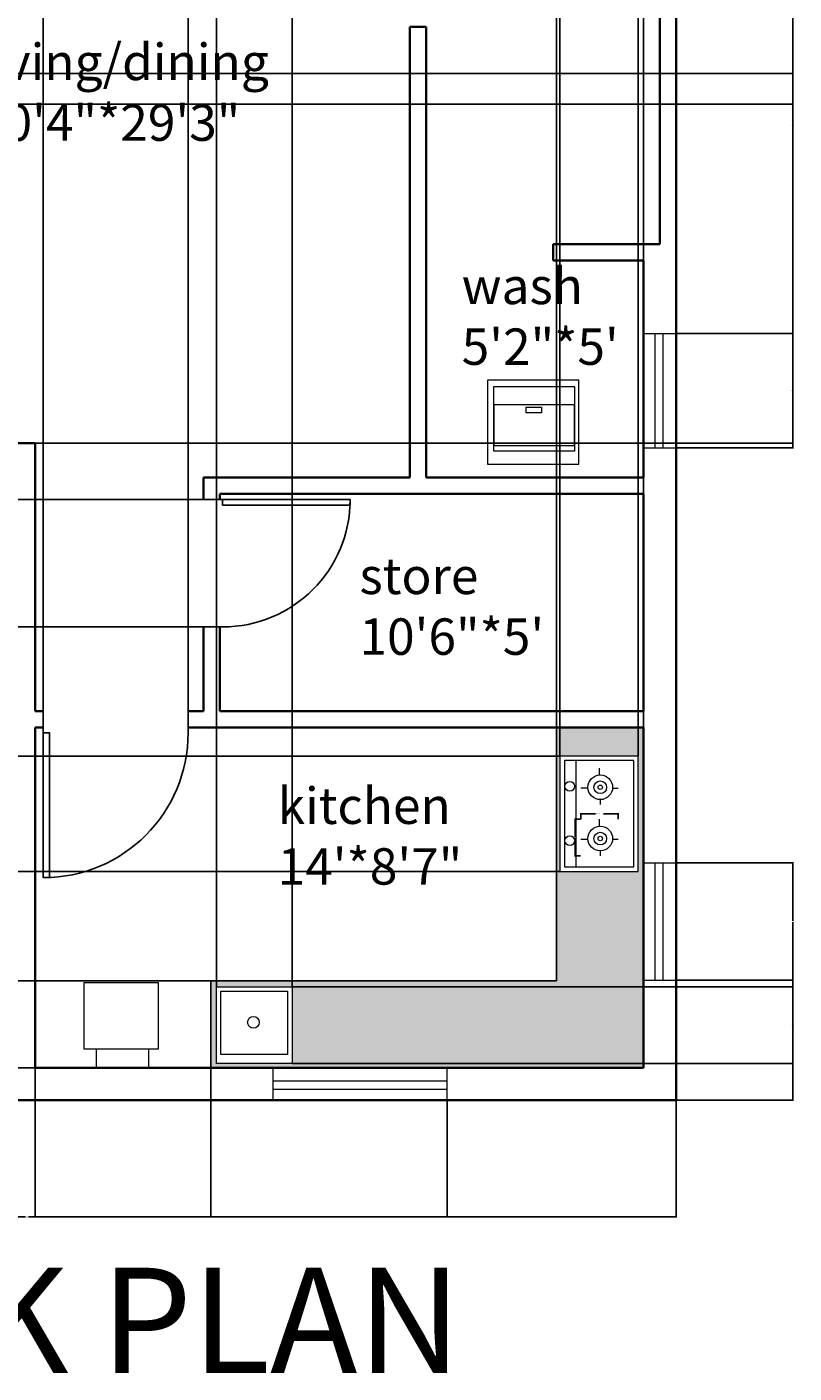
# Model space of a CAD drawing. Units: inches. Extents: x 2187 to 2611, y 763 to 1433.
# Tile 2 of 3: x 2399 to 2611, y 763 to 1135. Entities that reach past the tile are written whole.
import ezdxf

# ---------------------------------------------------------------- set-up
doc = ezdxf.new("R2010")
doc.units = ezdxf.units.IN
for name, color, linetype, lineweight in [('A-ANNO-DIMS', 2, 'Continuous', 18), ('A-ANNO-TITL', 7, 'Continuous', 35), ('A-AREA-IDEN', 7, 'Continuous', 18), ('A-EQPM', 82, 'Continuous', 18), ('A-FLOR-FIXT', 82, 'Continuous', 18), ('A-MILL-PATT', 11, 'Continuous', 13), ('A-WALL', 7, 'Continuous', 35), ('DOOR', 130, 'Continuous', 25), ('KITCHEN', 11, 'Continuous', 25), ('WINDOW', 50, 'Continuous', 20)]:
    doc.layers.add(name, color=color, linetype=linetype, lineweight=lineweight)
doc.styles.get("Standard").update_dxf_attribs({"font": 'arial.ttf'})
doc.dimstyles.get("Standard").update_dxf_attribs({"dimtxt": 0.18, "dimasz": 0.18, "dimexe": 0.18, "dimexo": 0.0625, "dimgap": 0.09, "dimtad": 0, "dimtih": 1, "dimtoh": 1, "dimdec": 4, "dimzin": 0, "dimdsep": 46, "dimtxsty": 'Standard', "dimcen": 0.09, "dimadec": 0, "dimazin": 0, "dimtfac": 1, "dimtdec": 4, "dimtofl": 0, "dimtmove": 0, "dimatfit": 3, "dimfxl": 1, "dimtolj": 1, "dimtzin": 0, "dimarcsym": 0})

# ---------------------------------------------------------------- blocks, each defined once
blk = doc.blocks.new('*U2')
for p, q in [((0, 0), (0, -6)), ((40, 0), (40, -6))]:
    blk.add_line(p, q)
blk.add_lwpolyline([(0, 0), (0, 40), (1.75, 40), (1.75, 0)], close=True)
blk.add_arc((0, 0), 40, 0, 90)
blk = doc.blocks.new('WIN-48IN')
for p, q in [((0, 0), (0, 9)), ((48, 0), (48, 9)), ((0, 5.37), (48, 5.37)), ((0, 3.09), (48, 3.09))]:
    blk.add_line(p, q)
blk = doc.blocks.new('COOKTOP-BURNER')
for p, q in [((5.18, 8.19), (5.18, 10.1)), ((1.99, 4.55), (0, 4.55)), ((8.79, 4.58), (10.33, 4.58)), ((5.34, 1.38), (5.34, 0))]:
    blk.add_line(p, q)
for radius in [3.41, 1.74, 0.617]:
    blk.add_circle((5.39, 4.79), radius)
blk = doc.blocks.new('*D12')
at = {"layer": 'A-ANNO-DIMS', "color": 0, "lineweight": -2, "transparency": 16777216}
for p, q in [((2551.93, 916.46), (2551.93, 918.13)), ((2552.11, 917.95), (2556.01, 917.95)), ((2562.08, 917.95), (2558.19, 917.95)), ((2562.26, 916.46), (2562.26, 918.13))]:
    blk.add_line(p, q, dxfattribs=at)
at = {"layer": 'A-ANNO-DIMS', "color": 0, "lineweight": 100, "transparency": 16777216}
for points in [[(2552.11, 917.98), (2552.11, 917.92), (2551.93, 917.95)], [(2562.08, 917.98), (2562.08, 917.92), (2562.26, 917.95)]]:
    blk.add_solid(points, dxfattribs=at)
at = {"layer": 'Defpoints', "color": 0, "lineweight": 100, "transparency": 16777216}
for p in [(2551.93, 916.4), (2562.26, 917.95), (2562.26, 916.4)]:
    blk.add_point(p, dxfattribs=at)
at = {"layer": 'A-ANNO-DIMS', "color": 0, "transparency": 16777216, "insert": (2557.1, 917.95), "char_height": 0.18, "attachment_point": 5}
blk.add_mtext('\\A1;BURNER 10 TYP.', dxfattribs=at)
blk = doc.blocks.new('*D13')
at = {"layer": 'A-ANNO-DIMS', "color": 0, "lineweight": -2, "transparency": 16777216}
for p, q in [((2551.87, 916.4), (2550.2, 916.4)), ((2550.38, 916.22), (2550.38, 911.53)), ((2550.38, 906.48), (2550.38, 911.17)), ((2551.87, 906.3), (2550.2, 906.3))]:
    blk.add_line(p, q, dxfattribs=at)
at = {"layer": 'A-ANNO-DIMS', "color": 0, "lineweight": 100, "transparency": 16777216}
for points in [[(2550.35, 916.22), (2550.41, 916.22), (2550.38, 916.4)], [(2550.35, 906.48), (2550.41, 906.48), (2550.38, 906.3)]]:
    blk.add_solid(points, dxfattribs=at)
at = {"layer": 'Defpoints', "color": 0, "lineweight": 100, "transparency": 16777216}
for p in [(2550.38, 916.4), (2551.93, 916.4), (2551.93, 906.3)]:
    blk.add_point(p, dxfattribs=at)
at = {"layer": 'A-ANNO-DIMS', "color": 0, "transparency": 16777216, "insert": (2550.38, 911.35), "char_height": 0.18, "attachment_point": 5}
blk.add_mtext('\\A1;10 TYP.', dxfattribs=at)
blk = doc.blocks.new('*D14')
at = {"layer": 'A-ANNO-DIMS', "color": 0, "lineweight": -2, "transparency": 16777216}
for p, q in [((2219.77, 838.73), (2219.77, 806.41)), ((2578.27, 838.73), (2578.27, 806.41)), ((2219.95, 806.59), (2398.62, 806.59)), ((2578.09, 806.59), (2399.41, 806.59))]:
    blk.add_line(p, q, dxfattribs=at)
at = {"layer": 'A-ANNO-DIMS', "color": 0, "lineweight": 100, "transparency": 16777216}
for points in [[(2219.95, 806.62), (2219.95, 806.56), (2219.77, 806.59)], [(2578.09, 806.62), (2578.09, 806.56), (2578.27, 806.59)]]:
    blk.add_solid(points, dxfattribs=at)
at = {"layer": 'Defpoints', "color": 0, "lineweight": 100, "transparency": 16777216}
for p in [(2219.77, 838.79), (2578.27, 838.79), (2578.27, 806.59)]:
    blk.add_point(p, dxfattribs=at)
at = {"layer": 'A-ANNO-DIMS', "color": 0, "transparency": 16777216, "insert": (2399.02, 806.59), "char_height": 0.18, "attachment_point": 5}
blk.add_mtext('\\A1;358.5', dxfattribs=at)
blk = doc.blocks.new('*D26')
at = {"layer": 'A-ANNO-DIMS', "color": 0, "lineweight": -2, "transparency": 16777216}
for p, q in [((2578.33, 1165.62), (2610.65, 1165.62)), ((2610.47, 1165.44), (2610.47, 1108.31)), ((2610.47, 1050.81), (2610.47, 1107.94)), ((2578.33, 1050.63), (2610.65, 1050.63))]:
    blk.add_line(p, q, dxfattribs=at)
at = {"layer": 'A-ANNO-DIMS', "color": 0, "lineweight": 100, "transparency": 16777216}
for points in [[(2610.44, 1165.44), (2610.5, 1165.44), (2610.47, 1165.62)], [(2610.44, 1050.81), (2610.5, 1050.81), (2610.47, 1050.63)]]:
    blk.add_solid(points, dxfattribs=at)
at = {"layer": 'Defpoints', "color": 0, "lineweight": 100, "transparency": 16777216}
for p in [(2578.27, 1165.62), (2610.47, 1165.62), (2578.27, 1050.63)]:
    blk.add_point(p, dxfattribs=at)
at = {"layer": 'A-ANNO-DIMS', "color": 0, "transparency": 16777216, "insert": (2610.47, 1108.13), "char_height": 0.18, "attachment_point": 5}
blk.add_mtext('\\A1;114.99', dxfattribs=at)
blk = doc.blocks.new('*D27')
at = {"layer": 'A-ANNO-DIMS', "color": 0, "lineweight": -2, "transparency": 16777216}
for p, q in [((2578.33, 1050.63), (2610.65, 1050.63)), ((2610.47, 1050.45), (2610.47, 1035.02)), ((2610.47, 1019.23), (2610.47, 1034.66)), ((2578.33, 1019.05), (2610.65, 1019.05))]:
    blk.add_line(p, q, dxfattribs=at)
at = {"layer": 'A-ANNO-DIMS', "color": 0, "lineweight": 100, "transparency": 16777216}
for points in [[(2610.44, 1050.45), (2610.5, 1050.45), (2610.47, 1050.63)], [(2610.44, 1019.23), (2610.5, 1019.23), (2610.47, 1019.05)]]:
    blk.add_solid(points, dxfattribs=at)
at = {"layer": 'Defpoints', "color": 0, "lineweight": 100, "transparency": 16777216}
for p in [(2578.27, 1050.63), (2610.47, 1050.63), (2578.27, 1019.05)]:
    blk.add_point(p, dxfattribs=at)
at = {"layer": 'A-ANNO-DIMS', "color": 0, "transparency": 16777216, "insert": (2610.47, 1034.84), "char_height": 0.18, "attachment_point": 5}
blk.add_mtext('\\A1;31.58', dxfattribs=at)
blk = doc.blocks.new('*D29')
at = {"layer": 'A-ANNO-DIMS', "color": 0, "lineweight": -2, "transparency": 16777216}
for p, q in [((2447.71, 1004.76), (2187.39, 1004.76)), ((2187.57, 1004.58), (2187.57, 987.33)), ((2187.57, 969.72), (2187.57, 986.97)), ((2447.71, 969.54), (2187.39, 969.54))]:
    blk.add_line(p, q, dxfattribs=at)
at = {"layer": 'A-ANNO-DIMS', "color": 0, "lineweight": 100, "transparency": 16777216}
for points in [[(2187.54, 1004.58), (2187.6, 1004.58), (2187.57, 1004.76)], [(2187.54, 969.72), (2187.6, 969.72), (2187.57, 969.54)]]:
    blk.add_solid(points, dxfattribs=at)
at = {"layer": 'Defpoints', "color": 0, "lineweight": 100, "transparency": 16777216}
for p in [(2187.57, 1004.76), (2447.77, 1004.76), (2447.77, 969.54)]:
    blk.add_point(p, dxfattribs=at)
at = {"layer": 'A-ANNO-DIMS', "color": 0, "transparency": 16777216, "insert": (2187.57, 987.15), "char_height": 0.18, "attachment_point": 5}
blk.add_mtext('\\A1;35.22', dxfattribs=at)
blk = doc.blocks.new('*D31')
at = {"layer": 'A-ANNO-DIMS', "color": 0, "lineweight": -2, "transparency": 16777216}
for p, q in [((2313.33, 1162.4), (2610.65, 1162.4)), ((2610.47, 1162.22), (2610.47, 1142.58)), ((2610.47, 1122.58), (2610.47, 1142.22)), ((2313.33, 1122.4), (2610.65, 1122.4))]:
    blk.add_line(p, q, dxfattribs=at)
at = {"layer": 'A-ANNO-DIMS', "color": 0, "lineweight": 100, "transparency": 16777216}
for points in [[(2610.44, 1162.22), (2610.5, 1162.22), (2610.47, 1162.4)], [(2610.44, 1122.58), (2610.5, 1122.58), (2610.47, 1122.4)]]:
    blk.add_solid(points, dxfattribs=at)
at = {"layer": 'Defpoints', "color": 0, "lineweight": 100, "transparency": 16777216}
for p in [(2313.27, 1162.4), (2610.47, 1162.4), (2313.27, 1122.4)]:
    blk.add_point(p, dxfattribs=at)
at = {"layer": 'A-ANNO-DIMS', "color": 0, "transparency": 16777216, "insert": (2610.47, 1142.4), "char_height": 0.18, "attachment_point": 5}
blk.add_mtext('\\A1;40', dxfattribs=at)
blk = doc.blocks.new('*D33')
at = {"layer": 'A-ANNO-DIMS', "color": 0, "lineweight": -2, "transparency": 16777216}
for p, q in [((2545.27, 941.86), (2545.27, 1433.34)), ((2545.45, 1433.16), (2557.05, 1433.16)), ((2569.09, 1433.16), (2557.49, 1433.16)), ((2569.27, 941.86), (2569.27, 1433.34))]:
    blk.add_line(p, q, dxfattribs=at)
at = {"layer": 'A-ANNO-DIMS', "color": 0, "lineweight": 100, "transparency": 16777216}
for points in [[(2545.45, 1433.19), (2545.45, 1433.13), (2545.27, 1433.16)], [(2569.09, 1433.19), (2569.09, 1433.13), (2569.27, 1433.16)]]:
    blk.add_solid(points, dxfattribs=at)
at = {"layer": 'Defpoints', "color": 0, "lineweight": 100, "transparency": 16777216}
for p in [(2569.27, 1433.16), (2545.27, 941.79), (2569.27, 941.79)]:
    blk.add_point(p, dxfattribs=at)
at = {"layer": 'A-ANNO-DIMS', "color": 0, "transparency": 16777216, "insert": (2557.27, 1433.16), "char_height": 0.18, "attachment_point": 5}
blk.add_mtext('\\A1;24', dxfattribs=at)
blk = doc.blocks.new('*D34')
at = {"layer": 'A-ANNO-DIMS', "color": 0, "lineweight": -2, "transparency": 16777216}
for p, q in [((2449.71, 871.79), (2187.39, 871.79)), ((2187.57, 871.61), (2187.57, 859.97)), ((2187.57, 847.97), (2187.57, 859.61)), ((2449.71, 847.79), (2187.39, 847.79))]:
    blk.add_line(p, q, dxfattribs=at)
at = {"layer": 'A-ANNO-DIMS', "color": 0, "lineweight": 100, "transparency": 16777216}
for points in [[(2187.54, 871.61), (2187.6, 871.61), (2187.57, 871.79)], [(2187.54, 847.97), (2187.6, 847.97), (2187.57, 847.79)]]:
    blk.add_solid(points, dxfattribs=at)
at = {"layer": 'Defpoints', "color": 0, "lineweight": 100, "transparency": 16777216}
for p in [(2187.57, 871.79), (2449.78, 871.79), (2449.78, 847.79)]:
    blk.add_point(p, dxfattribs=at)
at = {"layer": 'A-ANNO-DIMS', "color": 0, "transparency": 16777216, "insert": (2187.57, 859.79), "char_height": 0.18, "attachment_point": 5}
blk.add_mtext('\\A1;24', dxfattribs=at)
blk = doc.blocks.new('*D35')
at = {"layer": 'A-ANNO-DIMS', "color": 0, "lineweight": -2, "transparency": 16777216}
for p, q in [((2401.27, 847.73), (2401.27, 806.41)), ((2449.78, 847.73), (2449.78, 806.41)), ((2401.45, 806.59), (2425.14, 806.59)), ((2449.6, 806.59), (2425.9, 806.59))]:
    blk.add_line(p, q, dxfattribs=at)
at = {"layer": 'A-ANNO-DIMS', "color": 0, "lineweight": 100, "transparency": 16777216}
for points in [[(2401.45, 806.62), (2401.45, 806.56), (2401.27, 806.59)], [(2449.6, 806.62), (2449.6, 806.56), (2449.78, 806.59)]]:
    blk.add_solid(points, dxfattribs=at)
at = {"layer": 'Defpoints', "color": 0, "lineweight": 100, "transparency": 16777216}
for p in [(2401.27, 847.79), (2449.78, 847.79), (2449.78, 806.59)]:
    blk.add_point(p, dxfattribs=at)
at = {"layer": 'A-ANNO-DIMS', "color": 0, "transparency": 16777216, "insert": (2425.52, 806.59), "char_height": 0.18, "attachment_point": 5}
blk.add_mtext('\\A1;48.51', dxfattribs=at)
blk = doc.blocks.new('*D36')
at = {"layer": 'A-ANNO-DIMS', "color": 0, "lineweight": -2, "transparency": 16777216}
for p, q in [((2403.54, 946.36), (2403.54, 1433.34)), ((2403.72, 1433.16), (2423.32, 1433.16)), ((2443.36, 1433.16), (2423.76, 1433.16)), ((2443.54, 946.36), (2443.54, 1433.34))]:
    blk.add_line(p, q, dxfattribs=at)
at = {"layer": 'A-ANNO-DIMS', "color": 0, "lineweight": 100, "transparency": 16777216}
for points in [[(2403.72, 1433.19), (2403.72, 1433.13), (2403.54, 1433.16)], [(2443.36, 1433.19), (2443.36, 1433.13), (2443.54, 1433.16)]]:
    blk.add_solid(points, dxfattribs=at)
at = {"layer": 'Defpoints', "color": 0, "lineweight": 100, "transparency": 16777216}
for p in [(2443.54, 1433.16), (2403.54, 946.29), (2443.54, 946.29)]:
    blk.add_point(p, dxfattribs=at)
at = {"layer": 'A-ANNO-DIMS', "color": 0, "transparency": 16777216, "insert": (2423.54, 1433.16), "char_height": 0.18, "attachment_point": 5}
blk.add_mtext('\\A1;40', dxfattribs=at)
blk = doc.blocks.new('*D37')
at = {"layer": 'A-ANNO-DIMS', "color": 0, "lineweight": -2, "transparency": 16777216}
for p, q in [((2515.03, 838.73), (2515.03, 806.41)), ((2578.27, 838.73), (2578.27, 806.41)), ((2515.21, 806.59), (2546.26, 806.59)), ((2578.09, 806.59), (2547.04, 806.59))]:
    blk.add_line(p, q, dxfattribs=at)
at = {"layer": 'A-ANNO-DIMS', "color": 0, "lineweight": 100, "transparency": 16777216}
for points in [[(2515.21, 806.62), (2515.21, 806.56), (2515.03, 806.59)], [(2578.09, 806.62), (2578.09, 806.56), (2578.27, 806.59)]]:
    blk.add_solid(points, dxfattribs=at)
at = {"layer": 'Defpoints', "color": 0, "lineweight": 100, "transparency": 16777216}
for p in [(2515.03, 838.79), (2578.27, 838.79), (2578.27, 806.59)]:
    blk.add_point(p, dxfattribs=at)
at = {"layer": 'A-ANNO-DIMS', "color": 0, "transparency": 16777216, "insert": (2546.65, 806.59), "char_height": 0.18, "attachment_point": 5}
blk.add_mtext('\\A1;63.23', dxfattribs=at)
blk = doc.blocks.new('*D38')
at = {"layer": 'A-ANNO-DIMS', "color": 0, "lineweight": -2, "transparency": 16777216}
for p, q in [((2578.33, 871.93), (2610.65, 871.93)), ((2610.47, 871.75), (2610.47, 855.55)), ((2610.47, 838.97), (2610.47, 855.18)), ((2578.33, 838.79), (2610.65, 838.79))]:
    blk.add_line(p, q, dxfattribs=at)
at = {"layer": 'A-ANNO-DIMS', "color": 0, "lineweight": 100, "transparency": 16777216}
for points in [[(2610.44, 871.75), (2610.5, 871.75), (2610.47, 871.93)], [(2610.44, 838.97), (2610.5, 838.97), (2610.47, 838.79)]]:
    blk.add_solid(points, dxfattribs=at)
at = {"layer": 'Defpoints', "color": 0, "lineweight": 100, "transparency": 16777216}
for p in [(2578.27, 871.93), (2610.47, 871.93), (2578.27, 838.79)]:
    blk.add_point(p, dxfattribs=at)
at = {"layer": 'A-ANNO-DIMS', "color": 0, "transparency": 16777216, "insert": (2610.47, 855.36), "char_height": 0.18, "attachment_point": 5}
blk.add_mtext('\\A1;33.14', dxfattribs=at)
blk = doc.blocks.new('*D39')
at = {"layer": 'A-ANNO-DIMS', "color": 0, "lineweight": -2, "transparency": 16777216}
for p, q in [((2578.33, 904.34), (2610.65, 904.34)), ((2610.47, 904.16), (2610.47, 888.32)), ((2610.47, 872.11), (2610.47, 887.95)), ((2578.33, 871.93), (2610.65, 871.93))]:
    blk.add_line(p, q, dxfattribs=at)
at = {"layer": 'A-ANNO-DIMS', "color": 0, "lineweight": 100, "transparency": 16777216}
for points in [[(2610.44, 904.16), (2610.5, 904.16), (2610.47, 904.34)], [(2610.44, 872.11), (2610.5, 872.11), (2610.47, 871.93)]]:
    blk.add_solid(points, dxfattribs=at)
at = {"layer": 'Defpoints', "color": 0, "lineweight": 100, "transparency": 16777216}
for p in [(2578.27, 904.34), (2610.47, 904.34), (2578.27, 871.93)]:
    blk.add_point(p, dxfattribs=at)
at = {"layer": 'A-ANNO-DIMS', "color": 0, "transparency": 16777216, "insert": (2610.47, 888.14), "char_height": 0.18, "attachment_point": 5}
blk.add_mtext('\\A1;32.406', dxfattribs=at)
blk = doc.blocks.new('*D40')
at = {"layer": 'A-ANNO-DIMS', "color": 0, "lineweight": -2, "transparency": 16777216}
for p, q in [((2451.33, 870.16), (2451.33, 1433.34)), ((2451.51, 1433.16), (2461.34, 1433.16)), ((2472.1, 1433.16), (2462.27, 1433.16)), ((2472.28, 870.16), (2472.28, 1433.34))]:
    blk.add_line(p, q, dxfattribs=at)
at = {"layer": 'A-ANNO-DIMS', "color": 0, "lineweight": 100, "transparency": 16777216}
for points in [[(2451.51, 1433.19), (2451.51, 1433.13), (2451.33, 1433.16)], [(2472.1, 1433.19), (2472.1, 1433.13), (2472.28, 1433.16)]]:
    blk.add_solid(points, dxfattribs=at)
at = {"layer": 'Defpoints', "color": 0, "lineweight": 100, "transparency": 16777216}
for p in [(2472.28, 1433.16), (2451.33, 870.1), (2472.28, 870.1)]:
    blk.add_point(p, dxfattribs=at)
at = {"layer": 'A-ANNO-DIMS', "color": 0, "transparency": 16777216, "insert": (2461.81, 1433.16), "char_height": 0.18, "attachment_point": 5}
blk.add_mtext('\\A1;20.953', dxfattribs=at)
blk = doc.blocks.new('*D41')
at = {"layer": 'A-ANNO-DIMS', "color": 0, "lineweight": -2, "transparency": 16777216}
for p, q in [((2472.34, 870.1), (2610.65, 870.1)), ((2610.47, 869.92), (2610.47, 859.73)), ((2610.47, 849.17), (2610.47, 859.36)), ((2472.34, 848.99), (2610.65, 848.99))]:
    blk.add_line(p, q, dxfattribs=at)
at = {"layer": 'A-ANNO-DIMS', "color": 0, "lineweight": 100, "transparency": 16777216}
for points in [[(2610.44, 869.92), (2610.5, 869.92), (2610.47, 870.1)], [(2610.44, 849.17), (2610.5, 849.17), (2610.47, 848.99)]]:
    blk.add_solid(points, dxfattribs=at)
at = {"layer": 'Defpoints', "color": 0, "lineweight": 100, "transparency": 16777216}
for p in [(2472.28, 870.1), (2610.47, 870.1), (2472.28, 848.99)]:
    blk.add_point(p, dxfattribs=at)
at = {"layer": 'A-ANNO-DIMS', "color": 0, "transparency": 16777216, "insert": (2610.47, 859.54), "char_height": 0.18, "attachment_point": 5}
blk.add_mtext('\\A1;21.115', dxfattribs=at)
blk = doc.blocks.new('*D42')
at = {"layer": 'A-ANNO-DIMS', "color": 0, "lineweight": -2, "transparency": 16777216}
for p, q in [((2546.19, 933.93), (2546.19, 1433.34)), ((2546.37, 1433.16), (2556.61, 1433.16)), ((2567.64, 1433.16), (2557.4, 1433.16)), ((2567.82, 933.93), (2567.82, 1433.34))]:
    blk.add_line(p, q, dxfattribs=at)
at = {"layer": 'A-ANNO-DIMS', "color": 0, "lineweight": 100, "transparency": 16777216}
for points in [[(2546.37, 1433.19), (2546.37, 1433.13), (2546.19, 1433.16)], [(2567.64, 1433.19), (2567.64, 1433.13), (2567.82, 1433.16)]]:
    blk.add_solid(points, dxfattribs=at)
at = {"layer": 'Defpoints', "color": 0, "lineweight": 100, "transparency": 16777216}
for p in [(2567.82, 1433.16), (2546.19, 933.87), (2567.82, 933.87)]:
    blk.add_point(p, dxfattribs=at)
at = {"layer": 'A-ANNO-DIMS', "color": 0, "transparency": 16777216, "insert": (2557.01, 1433.16), "char_height": 0.18, "attachment_point": 5}
blk.add_mtext('\\A1;21.63', dxfattribs=at)
blk = doc.blocks.new('*D43')
at = {"layer": 'A-ANNO-DIMS', "color": 0, "lineweight": -2, "transparency": 16777216}
for p, q in [((2546.13, 933.87), (2187.39, 933.87)), ((2187.57, 933.69), (2187.57, 918.13)), ((2187.57, 902.21), (2187.57, 917.77)), ((2546.13, 902.03), (2187.39, 902.03))]:
    blk.add_line(p, q, dxfattribs=at)
at = {"layer": 'A-ANNO-DIMS', "color": 0, "lineweight": 100, "transparency": 16777216}
for points in [[(2187.54, 933.69), (2187.6, 933.69), (2187.57, 933.87)], [(2187.54, 902.21), (2187.6, 902.21), (2187.57, 902.03)]]:
    blk.add_solid(points, dxfattribs=at)
at = {"layer": 'Defpoints', "color": 0, "lineweight": 100, "transparency": 16777216}
for p in [(2187.57, 933.87), (2546.19, 933.87), (2546.19, 902.03)]:
    blk.add_point(p, dxfattribs=at)
at = {"layer": 'A-ANNO-DIMS', "color": 0, "transparency": 16777216, "insert": (2187.57, 917.95), "char_height": 0.18, "attachment_point": 5}
blk.add_mtext('\\A1;31.837', dxfattribs=at)
blk = doc.blocks.new('*D45')
at = {"layer": 'A-ANNO-DIMS', "color": 0, "lineweight": -2, "transparency": 16777216}
for p, q in [((2345.13, 1113.96), (2610.65, 1113.96)), ((2610.47, 1113.78), (2610.47, 1067.31)), ((2610.47, 1020.47), (2610.47, 1066.94)), ((2345.13, 1020.29), (2610.65, 1020.29))]:
    blk.add_line(p, q, dxfattribs=at)
at = {"layer": 'A-ANNO-DIMS', "color": 0, "lineweight": 100, "transparency": 16777216}
for points in [[(2610.44, 1113.78), (2610.5, 1113.78), (2610.47, 1113.96)], [(2610.44, 1020.47), (2610.5, 1020.47), (2610.47, 1020.29)]]:
    blk.add_solid(points, dxfattribs=at)
at = {"layer": 'Defpoints', "color": 0, "lineweight": 100, "transparency": 16777216}
for p in [(2345.07, 1113.96), (2610.47, 1113.96), (2345.07, 1020.29)]:
    blk.add_point(p, dxfattribs=at)
at = {"layer": 'A-ANNO-DIMS', "color": 0, "transparency": 16777216, "insert": (2610.47, 1067.13), "char_height": 0.18, "attachment_point": 5}
blk.add_mtext('\\A1;93.67', dxfattribs=at)

msp = doc.modelspace()

# ---------------------------------------------------------------- hatches: boundary and pattern name
at = {"layer": 'A-MILL-PATT'}
h = msp.add_hatch(color=256, dxfattribs=at)
h.dxf.hatch_style = 1
h.paths.add_polyline_path([(2569.2681, 941.7937), (2545.2681, 941.7937), (2545.2681, 887.4363), (2545.2681, 871.7937), (2449.7774, 871.7937), (2449.7774, 847.7937), (2569.2681, 847.7937)])
h.paths.add_polyline_path([(2472.2814, 848.9857), (2451.3286, 848.9857), (2451.3286, 870.1006), (2472.2814, 870.1006)], flags=16)
h.paths.add_polyline_path([(2470.9727, 851.422), (2452.546, 851.422), (2452.546, 868.9386), (2470.9727, 868.9386)], flags=0)
h.paths.add_polyline_path([(2546.1934, 902.0317), (2546.1934, 933.8683), (2567.8237, 933.8683), (2567.8237, 902.0317)], flags=16)
h.paths.add_polyline_path([(2547.449, 903.2873), (2547.449, 932.6128), (2566.5682, 932.6128), (2566.5682, 903.2873)], flags=0)
h.paths.add_polyline_path([(2459.9391, 860.3197, -1), (2463.1875, 860.3197, -1)], flags=0)
h.paths.add_polyline_path([(2547.5717, 910.5139, -1), (2550.27, 910.5139, -1)], flags=0)
h.paths.add_polyline_path([(2553.9157, 911.0895, -1), (2560.7314, 911.0895, -1)], flags=0)
h.paths.add_polyline_path([(2555.5839, 911.0895, -1), (2559.0633, 911.0895, -1)], flags=0)
h.paths.add_polyline_path([(2556.7066, 911.0895, -1), (2557.9405, 911.0895, -1)], flags=0)
h.paths.add_polyline_path([(2547.5717, 925.5242, -1), (2550.27, 925.5242, -1)], flags=0)
h.paths.add_polyline_path([(2553.9157, 925.259, -1), (2560.7314, 925.259, -1)], flags=0)
h.paths.add_polyline_path([(2555.5839, 925.259, -1), (2559.0633, 925.259, -1)], flags=0)
h.paths.add_polyline_path([(2556.7066, 925.259, -1), (2557.9405, 925.259, -1)], flags=0)

# ---------------------------------------------------------------- linework, layer by layer
at = {"layer": 'A-EQPM'}
msp.add_line((2550.5454, 932.6128), (2550.5454, 903.2873), dxfattribs=at)
for points in [[(2526.2088, 1014.5087), (2551.4027, 1014.5087), (2551.4027, 1037.6913), (2526.2088, 1037.6913)], [(2527.9169, 1035.9846), (2550.1793, 1035.9846), (2550.1793, 1018.0643), (2527.9169, 1018.0643)], [(2527.9169, 1019.6918), (2550.1793, 1019.6918), (2550.1793, 1030.9359), (2527.9169, 1030.9359)], [(2536.8927, 1030.2614), (2541.0736, 1030.2614), (2541.0736, 1028.7017), (2536.8927, 1028.7017)], [(2567.8237, 933.8683), (2546.1934, 933.8683), (2546.1934, 902.0317), (2567.8237, 902.0317)], [(2566.5682, 932.6128), (2547.449, 932.6128), (2547.449, 903.2873), (2566.5682, 903.2873)], [(2414.752, 852.9676), (2435.3384, 852.9676), (2435.3384, 871.2519), (2414.752, 871.2519)], [(2418.1831, 852.9676), (2432.6221, 852.9676), (2432.6221, 847.7937), (2418.1831, 847.7937)]]:
    msp.add_lwpolyline(points, close=True, dxfattribs=at)
for centre, radius in [((2548.9208, 925.5242), 1.3492), ((2548.9208, 910.5139), 1.3492), ((2557.3236, 911.0895), 3.4079)]:
    msp.add_circle(centre, radius, dxfattribs=at)
at = {"layer": 'A-FLOR-FIXT'}
for points in [[(2451.3286, 870.1006), (2472.2814, 870.1006), (2472.2814, 848.9857), (2451.3286, 848.9857)], [(2452.546, 868.9386), (2470.9727, 868.9386), (2470.9727, 851.422), (2452.546, 851.422)]]:
    msp.add_lwpolyline(points, close=True, dxfattribs=at)
msp.add_circle((2461.5633, 860.3197), 1.6242, dxfattribs=at)
at = {"layer": 'A-WALL'}
for p, q in [((2573.7681, 1075.2937), (2573.7681, 1275.4602)), ((2578.2681, 1075.2937), (2578.2681, 1275.4602)), ((2504.7681, 1103.3659), (2504.7681, 1135.278)), ((2504.7681, 1135.278), (2509.2681, 1135.278)), ((2509.2681, 1135.278), (2509.2681, 1103.3659)), ((2504.7681, 1010.7937), (2504.7681, 1103.3659)), ((2509.2681, 1010.7937), (2509.2681, 1103.3659)), ((2573.7681, 1075.2937), (2544.3479, 1075.2937)), ((2544.3479, 1075.2937), (2544.3479, 1070.7937)), ((2578.2681, 1010.7937), (2578.2681, 1075.2937)), ((2509.2681, 1070.7937), (2509.2681, 1010.7937)), ((2569.2681, 1070.7937), (2544.3479, 1070.7937)), ((2569.2681, 1010.7937), (2569.2681, 1070.7937)), ((2389.6096, 1020.2937), (2401.2681, 1020.2937)), ((2401.2681, 946.2937), (2401.2681, 1020.2937)), ((2447.7681, 1010.7937), (2447.7681, 1004.7585)), ((2504.7681, 1010.7937), (2447.7681, 1010.7937)), ((2569.2681, 1010.7937), (2509.2681, 1010.7937)), ((2578.2681, 1006.2937), (2578.2681, 1010.7937)), ((2569.2681, 1006.2937), (2452.2681, 1006.2937)), ((2452.2681, 1006.2937), (2452.2681, 1004.7585)), ((2569.2681, 946.2937), (2569.2681, 1006.2937)), ((2578.2681, 946.2937), (2578.2681, 1006.2937)), ((2447.7681, 969.5415), (2447.7681, 946.2937)), ((2452.2681, 969.5415), (2452.2681, 946.2937)), ((2403.5404, 946.2937), (2401.2681, 946.2937)), ((2447.7681, 946.2937), (2443.5404, 946.2937)), ((2569.2681, 946.2937), (2452.2681, 946.2937)), ((2578.2681, 941.7937), (2578.2681, 946.2937)), ((2401.2681, 847.7937), (2401.2681, 941.7937)), ((2403.5404, 941.7937), (2401.2681, 941.7937)), ((2569.2681, 941.7937), (2443.5404, 941.7937)), ((2569.2681, 847.7937), (2569.2681, 941.7937)), ((2578.2681, 838.7937), (2578.2681, 941.7937)), ((2401.2681, 847.7937), (2569.2681, 847.7937)), ((2219.7681, 838.7937), (2401.2681, 838.7937)), ((2401.2681, 838.7937), (2569.2681, 838.7937)), ((2569.2681, 838.7937), (2578.2681, 838.7937))]:
    msp.add_line(p, q, dxfattribs=at)
at = {"layer": 'KITCHEN'}
for p, q in [((2569.2681, 941.7937), (2545.2681, 941.7937)), ((2545.2681, 941.7937), (2545.2681, 887.4363)), ((2545.2681, 871.7937), (2545.2681, 891.0213)), ((2449.7774, 847.7937), (2449.7774, 871.7937)), ((2449.7774, 871.7937), (2545.2681, 871.7937))]:
    msp.add_line(p, q, dxfattribs=at)
at = {"layer": 'WINDOW'}
for p, q in [((2569.2681, 1050.6332), (2578.2681, 1050.6332)), ((2572.3628, 1050.6332), (2572.3628, 1019.0505)), ((2574.6351, 1050.6332), (2574.6351, 1019.0505)), ((2569.2681, 1019.0505), (2578.2681, 1019.0505)), ((2569.2681, 904.3401), (2578.2681, 904.3401)), ((2572.3628, 904.3401), (2572.3628, 871.9337)), ((2574.6351, 904.3401), (2574.6351, 871.9337)), ((2569.2681, 871.9337), (2578.2681, 871.9337))]:
    msp.add_line(p, q, dxfattribs=at)

# ---------------------------------------------------------------- block references
at = {"layer": 'A-EQPM'}
for p in [(2551.9335, 920.4685), (2551.9335, 906.299)]:
    msp.add_blockref('COOKTOP-BURNER', p, dxfattribs=at)
at = {"layer": 'DOOR', "xscale": 0.8804235154867445, "yscale": 0.8804235154867445, "zscale": 0.8804235154867445, "rotation": 270}
msp.add_blockref('*U2', (2453.0506, 1004.7585), dxfattribs=at)
at = {"layer": 'DOOR', "xscale": -1, "rotation": 180}
msp.add_blockref('*U2', (2403.5404, 940.2937), dxfattribs=at)
at = {"layer": 'WINDOW'}
msp.add_blockref('WIN-48IN', (2467.0332, 838.7937), dxfattribs=at)

# ---------------------------------------------------------------- texts
at = {"layer": 'A-ANNO-TITL', "insert": (2299.0368, 792.5375), "char_height": 29.09468, "attachment_point": 1}
msp.add_mtext_dynamic_manual_height_columns('2 BHK PLAN', width=464.084837, gutter_width=145.4734, heights=[0], dxfattribs=at)
at = {"layer": 'A-AREA-IDEN', "attachment_point": 1}
for s, insert, char_height in [('living/dining\\P10\'4"*29\'3"', (2385.2182, 1130.6372), 10.056757), ('\\pxt8;wash\\P\\ptz;5\'2"*5\'', (2519.0611, 1068.7545), 10.056757), ('\\pxt8;store\\P\\ptz;10\'6"*5\'', (2490.8403, 988.6661), 10.056757), ('kitchen\\P14\'*8\'7"', (2468.2341, 925.183), 10.05676)]:
    msp.add_mtext_dynamic_manual_height_columns(s, width=160.413815, gutter_width=50.2838, heights=[0], dxfattribs=dict(at, insert=insert, char_height=char_height))

# ---------------------------------------------------------------- dimensions: what is measured, and where the dimension line sits
at = {"layer": 'A-ANNO-DIMS'}
for base, p1, p2, override, picture, middle in [((2443.5404, 1433.1602), (2403.5404, 946.2937), (2443.5404, 946.2937), {"dimdec": 0, "dimlfac": 1, "dimrnd": 0, "dimzin": 0, "dimdsep": 46, "dimlunit": 2}, '*D36', (2423.5404, 1433.1602)), ((2472.2814, 1433.1602), (2451.3286, 870.1006), (2472.2814, 870.1006), {"dimdec": 3, "dimlfac": 1, "dimrnd": 0, "dimzin": 0, "dimdsep": 46, "dimlunit": 2}, '*D40', (2461.805, 1433.1602)), ((2569.2681, 1433.1602), (2545.2681, 941.7937), (2569.2681, 941.7937), {"dimdec": 0, "dimlfac": 1, "dimrnd": 0, "dimzin": 0, "dimdsep": 46, "dimlunit": 2}, '*D33', (2557.2681, 1433.1602)), ((2567.8237, 1433.1602), (2546.1934, 933.8683), (2567.8237, 933.8683), {"dimdec": 2, "dimlfac": 1, "dimrnd": 0, "dimzin": 0, "dimdsep": 46, "dimlunit": 2}, '*D42', (2557.0086, 1433.1602)), ((2449.7774, 806.5937), (2401.2681, 847.7937), (2449.7774, 847.7937), {"dimdec": 2, "dimlfac": 1, "dimrnd": 0, "dimzin": 0, "dimdsep": 46, "dimlunit": 2}, '*D35', (2425.5227, 806.5937)), ((2578.2681, 806.5937), (2219.7681, 838.7937), (2578.2681, 838.7937), {"dimdec": 1, "dimlfac": 1, "dimrnd": 0, "dimzin": 0, "dimdsep": 46, "dimlunit": 2}, '*D14', (2399.0181, 806.5937)), ((2578.2681, 806.5937), (2515.0332, 838.7937), (2578.2681, 838.7937), {"dimdec": 2, "dimlfac": 1, "dimrnd": 0, "dimzin": 0, "dimdsep": 46, "dimlunit": 2}, '*D37', (2546.6506, 806.5937))]:
    dim = msp.add_linear_dim(base=base, p1=p1, p2=p2, dimstyle='Standard', override=override, dxfattribs=at)
    dim.commit()
    dim.dimension.update_dxf_attribs({"geometry": picture, "text_midpoint": middle})
for base, p1, p2, override, picture, middle in [((2610.4681, 1165.6205), (2578.2681, 1050.6332), (2578.2681, 1165.6205), {"dimdec": 2, "dimlfac": 1, "dimrnd": 0, "dimzin": 0, "dimdsep": 46, "dimlunit": 2}, '*D26', (2610.4681, 1108.1268)), ((2610.4681, 1162.3972), (2313.2681, 1122.3972), (2313.2681, 1162.3972), {"dimdec": 0, "dimlfac": 1, "dimrnd": 0, "dimzin": 0, "dimdsep": 46, "dimlunit": 2}, '*D31', (2610.4681, 1142.3972)), ((2610.4681, 1113.9602), (2345.0663, 1020.2937), (2345.0663, 1113.9602), {"dimdec": 2, "dimlfac": 1, "dimrnd": 0, "dimzin": 0, "dimdsep": 46, "dimlunit": 2}, '*D45', (2610.4681, 1067.127)), ((2610.4681, 1050.6332), (2578.2681, 1019.0505), (2578.2681, 1050.6332), {"dimdec": 2, "dimlfac": 1, "dimrnd": 0, "dimzin": 0, "dimdsep": 46, "dimlunit": 2}, '*D27', (2610.4681, 1034.8418)), ((2187.5681, 1004.7585), (2447.7681, 969.5415), (2447.7681, 1004.7585), {"dimdec": 2, "dimlfac": 1, "dimrnd": 0, "dimzin": 0, "dimdsep": 46, "dimlunit": 2}, '*D29', (2187.5681, 987.15)), ((2187.5681, 933.8683), (2546.1934, 902.0317), (2546.1934, 933.8683), {"dimdec": 3, "dimlfac": 1, "dimrnd": 0, "dimzin": 0, "dimdsep": 46, "dimlunit": 2}, '*D43', (2187.5681, 917.95)), ((2610.4681, 904.3401), (2578.2681, 871.9337), (2578.2681, 904.3401), {"dimdec": 3, "dimlfac": 1, "dimrnd": 0, "dimzin": 0, "dimdsep": 46, "dimlunit": 2}, '*D39', (2610.4681, 888.1369)), ((2187.5681, 871.7937), (2449.7774, 847.7937), (2449.7774, 871.7937), {"dimdec": 0, "dimlfac": 1, "dimrnd": 0, "dimzin": 0, "dimdsep": 46, "dimlunit": 2}, '*D34', (2187.5681, 859.7937)), ((2610.4681, 870.1006), (2472.2814, 848.9857), (2472.2814, 870.1006), {"dimdec": 3, "dimlfac": 1, "dimrnd": 0, "dimzin": 0, "dimdsep": 46, "dimlunit": 2}, '*D41', (2610.4681, 859.5431)), ((2610.4681, 871.9337), (2578.2681, 838.7937), (2578.2681, 871.9337), {"dimdec": 2, "dimlfac": 1, "dimrnd": 0, "dimzin": 0, "dimdsep": 46, "dimlunit": 2}, '*D38', (2610.4681, 855.3637))]:
    dim = msp.add_linear_dim(base=base, p1=p1, p2=p2, angle=90, dimstyle='Standard', override=override, dxfattribs=at)
    dim.commit()
    dim.dimension.update_dxf_attribs({"geometry": picture, "text_midpoint": middle})
dim = msp.add_linear_dim(base=(2550.3841, 916.3961), p1=(2551.9335, 906.299), p2=(2551.9335, 916.3961), angle=90, text='<> TYP.', dimstyle='Standard', override={"dimdec": 0, "dimlfac": 1, "dimrnd": 0, "dimzin": 0, "dimdsep": 46, "dimlunit": 2}, dxfattribs=at)
dim.commit()
dim.dimension.update_dxf_attribs({"geometry": '*D13', "text_midpoint": (2550.3841, 911.3476)})
dim = msp.add_linear_dim(base=(2562.2633, 917.9456), p1=(2551.9335, 916.3961), p2=(2562.2633, 916.3961), text='BURNER <> TYP.', dimstyle='Standard', override={"dimdec": 0, "dimlfac": 1, "dimrnd": 0, "dimzin": 0, "dimdsep": 46, "dimlunit": 2}, dxfattribs=at)
dim.commit()
dim.dimension.update_dxf_attribs({"geometry": '*D12', "text_midpoint": (2557.0984, 917.9456)})

doc.saveas('drawing.dxf')
